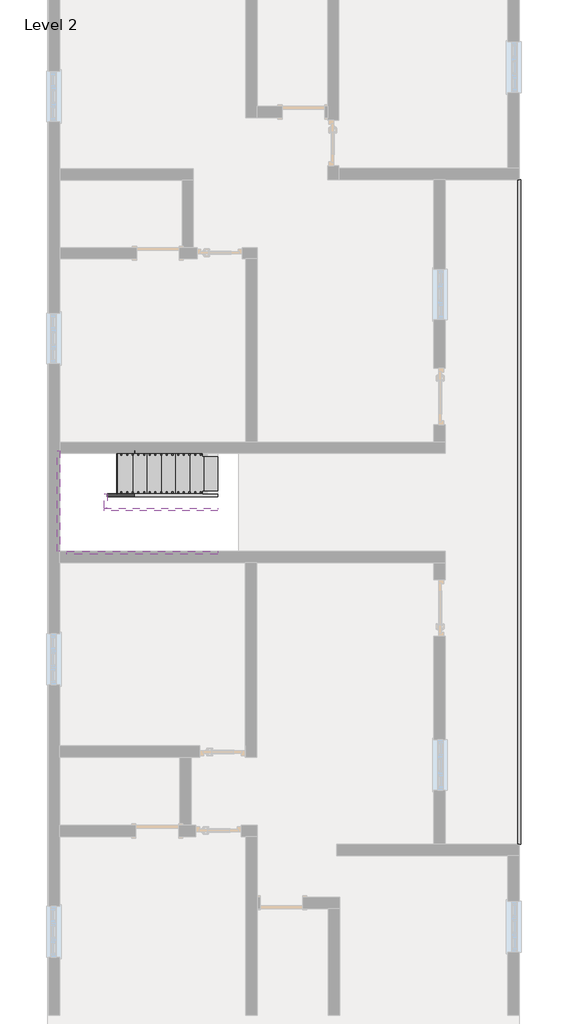
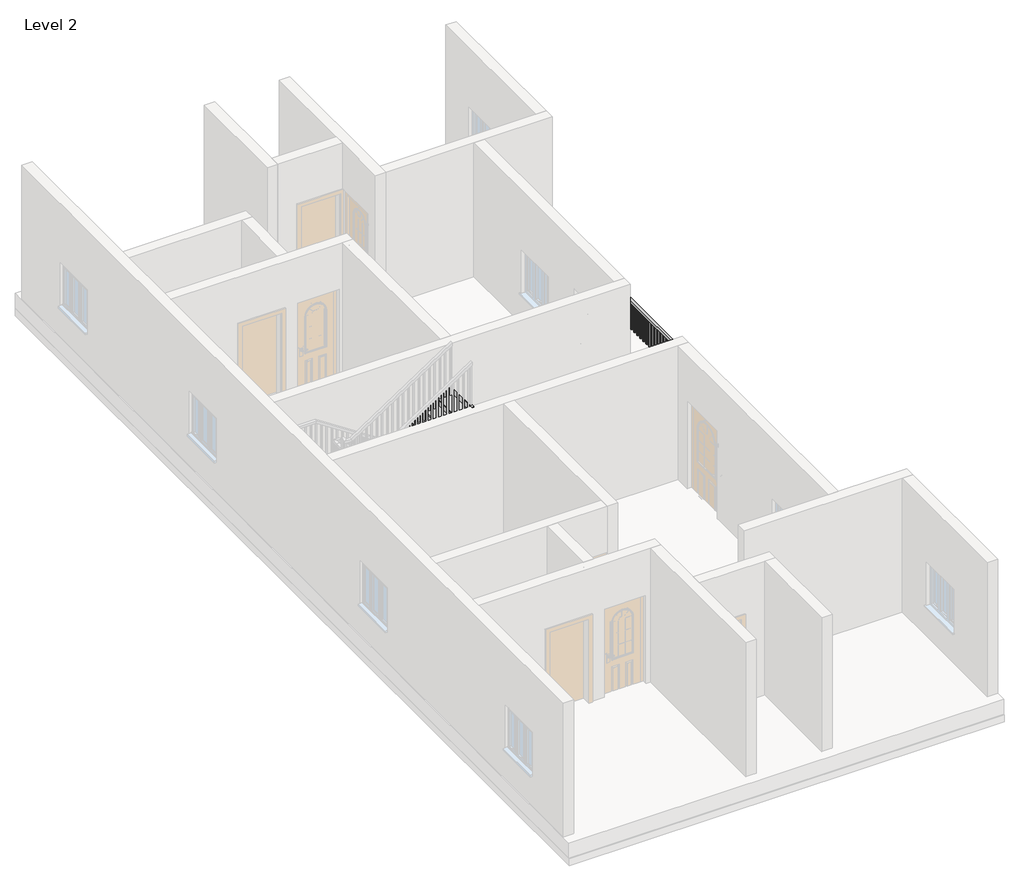
# One storey, part 3 of 3: 6 members, 1 railing, 1 stair flight.
"""IFC4 building model written with IfcOpenShell, lengths in millimetres."""

from ifc_helpers import new_model, si_unit, frame, origin, place, context, project, spatial, polyline, outline, extrude, transform, mapped, element, save
from components import stair_flight_1a1858fe

model = new_model("IFC4")

# Units and contexts
model_context = context("Model", 3, world=origin())
ifc_project = project(units=[si_unit("LENGTHUNIT", "METRE", prefix="MILLI")], contexts=[model_context])

# Site, building, storey
site = spatial("IfcSite", under=ifc_project)
building = spatial("IfcBuilding", under=site)
storey = spatial("IfcBuildingStorey", under=building, Name="Level 2", Elevation=3048.0)

# Members
placement = place(None, origin())
element("IfcMember", 1, ObjectType="Stringer - 2\" Width", at=placement, inside=storey, context=model_context, shape_type="SweptSolid", body=[
    extrude(outline(polyline([(3048.0, -2118.1728655), (3265.4747739, -2118.1728655), (4575.2681072, -4099.3728655), (4209.8806735, -4099.3728655), (3048.0, -2341.9063005), (3048.0, -2118.1728655)])), frame((0.0, 417.8797121, 0.0), z_axis=(0.0, 1.0, 0.0), x_axis=(0.0, 0.0, 1.0)), (0.0, 0.0, 1.0), 50.8),
])
element("IfcMember", 2, ObjectType="Stringer - 2\" Width", at=placement, inside=storey, context=model_context, shape_type="SweptSolid", body=[
    extrude(outline(polyline([(-4150.1728655, 468.6797121), (-4099.3728655, 468.6797121), (-4099.3728655, 214.6797121), (-4150.1728655, 214.6797121), (-4150.1728655, 468.6797121)])), frame((0.0, 0.0, 4330.7), z_axis=(0.0, 0.0, 1.0), x_axis=(1.0, 0.0, 0.0)), (0.0, 0.0, 1.0), 304.8),
])
element("IfcMember", 3, ObjectType="Stringer - 2\" Width", at=placement, inside=storey, context=model_context, shape_type="SweptSolid", body=[
    extrude(outline(polyline([(4776.7747739, -4150.1728655), (4411.3873402, -4150.1728655), (5754.765118, -2118.1728655), (6120.1525517, -2118.1728655), (4776.7747739, -4150.1728655)])), frame((0.0, 163.8797121, 0.0), z_axis=(0.0, 1.0, 0.0), x_axis=(0.0, 0.0, 1.0)), (0.0, 0.0, 1.0), 50.8),
])
element("IfcMember", 4, ObjectType="Stringer - 2\" Width", at=placement, inside=storey, context=model_context, shape_type="SweptSolid", body=[
    extrude(outline(polyline([(3048.0, -2118.1728655), (3265.4747739, -2118.1728655), (4635.5, -4190.4799301), (4635.5, -4743.1668047), (3048.0, -2341.9063005), (3048.0, -2118.1728655)])), frame((0.0, 1192.5797121, 0.0), z_axis=(0.0, 1.0, 0.0), x_axis=(0.0, 0.0, 1.0)), (0.0, 0.0, 1.0), 50.8),
])
element("IfcMember", 5, ObjectType="Stringer - 2\" Width", at=placement, inside=storey, context=model_context, shape_type="SweptSolid", body=[
    extrude(outline(polyline([(-4994.7394105, 1243.3797121), (-4943.9394105, 1243.3797121), (-4943.9394105, -560.0202879), (-4994.7394105, -560.0202879), (-4994.7394105, 1243.3797121)])), frame((0.0, 0.0, 4330.7), z_axis=(0.0, 0.0, 1.0), x_axis=(1.0, 0.0, 0.0)), (0.0, 0.0, 1.0), 304.8),
])
element("IfcMember", 6, ObjectType="Stringer - 2\" Width", at=placement, inside=storey, context=model_context, shape_type="SweptSolid", body=[
    extrude(outline(polyline([(4330.7, -4272.2209431), (5754.765118, -2118.1728655), (6120.1525517, -2118.1728655), (4330.7, -4824.9078176), (4330.7, -4272.2209431)])), frame((0.0, -610.8202879, 0.0), z_axis=(0.0, 1.0, 0.0), x_axis=(0.0, 0.0, 1.0)), (0.0, 0.0, 1.0), 50.8),
])

# Railing
element("IfcRailing", 7, ObjectType="Handrail - Rectangular", at=placement, inside=storey, context=model_context, shape_type="SweptSolid", body=[
    extrude(outline(polyline([(3298.3605895, -5805.1202879), (3247.5605895, -5805.1202879), (3247.5605895, 6094.2483916), (3298.3605895, 6094.2483916), (3298.3605895, -5805.1202879)])), frame((0.0, 0.0, 3911.6), z_axis=(0.0, 0.0, 1.0), x_axis=(1.0, 0.0, 0.0)), (0.0, 0.0, 1.0), 50.8),
    extrude(outline(polyline([(3282.4855895, 6072.5547121), (3263.4355895, 6072.5547121), (3263.4355895, 6091.6047121), (3282.4855895, 6091.6047121), (3282.4855895, 6072.5547121)])), frame((0.0, 0.0, 3048.0), z_axis=(0.0, 0.0, 1.0), x_axis=(1.0, 0.0, 0.0)), (0.0, 0.0, 1.0), 863.6),
    extrude(outline(polyline([(3282.4855895, 5970.9547121), (3263.4355895, 5970.9547121), (3263.4355895, 5990.0047121), (3282.4855895, 5990.0047121), (3282.4855895, 5970.9547121)])), frame((0.0, 0.0, 3048.0), z_axis=(0.0, 0.0, 1.0), x_axis=(1.0, 0.0, 0.0)), (0.0, 0.0, 1.0), 863.6),
    extrude(outline(polyline([(3282.4855895, 5869.3547121), (3263.4355895, 5869.3547121), (3263.4355895, 5888.4047121), (3282.4855895, 5888.4047121), (3282.4855895, 5869.3547121)])), frame((0.0, 0.0, 3048.0), z_axis=(0.0, 0.0, 1.0), x_axis=(1.0, 0.0, 0.0)), (0.0, 0.0, 1.0), 863.6),
    extrude(outline(polyline([(3282.4855895, 5767.7547121), (3263.4355895, 5767.7547121), (3263.4355895, 5786.8047121), (3282.4855895, 5786.8047121), (3282.4855895, 5767.7547121)])), frame((0.0, 0.0, 3048.0), z_axis=(0.0, 0.0, 1.0), x_axis=(1.0, 0.0, 0.0)), (0.0, 0.0, 1.0), 863.6),
    extrude(outline(polyline([(3282.4855895, 5666.1547121), (3263.4355895, 5666.1547121), (3263.4355895, 5685.2047121), (3282.4855895, 5685.2047121), (3282.4855895, 5666.1547121)])), frame((0.0, 0.0, 3048.0), z_axis=(0.0, 0.0, 1.0), x_axis=(1.0, 0.0, 0.0)), (0.0, 0.0, 1.0), 863.6),
    extrude(outline(polyline([(3282.4855895, 5564.5547121), (3263.4355895, 5564.5547121), (3263.4355895, 5583.6047121), (3282.4855895, 5583.6047121), (3282.4855895, 5564.5547121)])), frame((0.0, 0.0, 3048.0), z_axis=(0.0, 0.0, 1.0), x_axis=(1.0, 0.0, 0.0)), (0.0, 0.0, 1.0), 863.6),
    extrude(outline(polyline([(3282.4855895, 5462.9547121), (3263.4355895, 5462.9547121), (3263.4355895, 5482.0047121), (3282.4855895, 5482.0047121), (3282.4855895, 5462.9547121)])), frame((0.0, 0.0, 3048.0), z_axis=(0.0, 0.0, 1.0), x_axis=(1.0, 0.0, 0.0)), (0.0, 0.0, 1.0), 863.6),
    extrude(outline(polyline([(3282.4855895, 5361.3547121), (3263.4355895, 5361.3547121), (3263.4355895, 5380.4047121), (3282.4855895, 5380.4047121), (3282.4855895, 5361.3547121)])), frame((0.0, 0.0, 3048.0), z_axis=(0.0, 0.0, 1.0), x_axis=(1.0, 0.0, 0.0)), (0.0, 0.0, 1.0), 863.6),
    extrude(outline(polyline([(3282.4855895, 5259.7547121), (3263.4355895, 5259.7547121), (3263.4355895, 5278.8047121), (3282.4855895, 5278.8047121), (3282.4855895, 5259.7547121)])), frame((0.0, 0.0, 3048.0), z_axis=(0.0, 0.0, 1.0), x_axis=(1.0, 0.0, 0.0)), (0.0, 0.0, 1.0), 863.6),
    extrude(outline(polyline([(3282.4855895, 5158.1547121), (3263.4355895, 5158.1547121), (3263.4355895, 5177.2047121), (3282.4855895, 5177.2047121), (3282.4855895, 5158.1547121)])), frame((0.0, 0.0, 3048.0), z_axis=(0.0, 0.0, 1.0), x_axis=(1.0, 0.0, 0.0)), (0.0, 0.0, 1.0), 863.6),
    extrude(outline(polyline([(3282.4855895, 5056.5547121), (3263.4355895, 5056.5547121), (3263.4355895, 5075.6047121), (3282.4855895, 5075.6047121), (3282.4855895, 5056.5547121)])), frame((0.0, 0.0, 3048.0), z_axis=(0.0, 0.0, 1.0), x_axis=(1.0, 0.0, 0.0)), (0.0, 0.0, 1.0), 863.6),
    extrude(outline(polyline([(3282.4855895, 4954.9547121), (3263.4355895, 4954.9547121), (3263.4355895, 4974.0047121), (3282.4855895, 4974.0047121), (3282.4855895, 4954.9547121)])), frame((0.0, 0.0, 3048.0), z_axis=(0.0, 0.0, 1.0), x_axis=(1.0, 0.0, 0.0)), (0.0, 0.0, 1.0), 863.6),
    extrude(outline(polyline([(3282.4855895, 4853.3547121), (3263.4355895, 4853.3547121), (3263.4355895, 4872.4047121), (3282.4855895, 4872.4047121), (3282.4855895, 4853.3547121)])), frame((0.0, 0.0, 3048.0), z_axis=(0.0, 0.0, 1.0), x_axis=(1.0, 0.0, 0.0)), (0.0, 0.0, 1.0), 863.6),
    extrude(outline(polyline([(3282.4855895, 4751.7547121), (3263.4355895, 4751.7547121), (3263.4355895, 4770.8047121), (3282.4855895, 4770.8047121), (3282.4855895, 4751.7547121)])), frame((0.0, 0.0, 3048.0), z_axis=(0.0, 0.0, 1.0), x_axis=(1.0, 0.0, 0.0)), (0.0, 0.0, 1.0), 863.6),
    extrude(outline(polyline([(3282.4855895, 4650.1547121), (3263.4355895, 4650.1547121), (3263.4355895, 4669.2047121), (3282.4855895, 4669.2047121), (3282.4855895, 4650.1547121)])), frame((0.0, 0.0, 3048.0), z_axis=(0.0, 0.0, 1.0), x_axis=(1.0, 0.0, 0.0)), (0.0, 0.0, 1.0), 863.6),
    extrude(outline(polyline([(3282.4855895, 4548.5547121), (3263.4355895, 4548.5547121), (3263.4355895, 4567.6047121), (3282.4855895, 4567.6047121), (3282.4855895, 4548.5547121)])), frame((0.0, 0.0, 3048.0), z_axis=(0.0, 0.0, 1.0), x_axis=(1.0, 0.0, 0.0)), (0.0, 0.0, 1.0), 863.6),
    extrude(outline(polyline([(3282.4855895, 4446.9547121), (3263.4355895, 4446.9547121), (3263.4355895, 4466.0047121), (3282.4855895, 4466.0047121), (3282.4855895, 4446.9547121)])), frame((0.0, 0.0, 3048.0), z_axis=(0.0, 0.0, 1.0), x_axis=(1.0, 0.0, 0.0)), (0.0, 0.0, 1.0), 863.6),
    extrude(outline(polyline([(3282.4855895, 4345.3547121), (3263.4355895, 4345.3547121), (3263.4355895, 4364.4047121), (3282.4855895, 4364.4047121), (3282.4855895, 4345.3547121)])), frame((0.0, 0.0, 3048.0), z_axis=(0.0, 0.0, 1.0), x_axis=(1.0, 0.0, 0.0)), (0.0, 0.0, 1.0), 863.6),
    extrude(outline(polyline([(3282.4855895, 4243.7547121), (3263.4355895, 4243.7547121), (3263.4355895, 4262.8047121), (3282.4855895, 4262.8047121), (3282.4855895, 4243.7547121)])), frame((0.0, 0.0, 3048.0), z_axis=(0.0, 0.0, 1.0), x_axis=(1.0, 0.0, 0.0)), (0.0, 0.0, 1.0), 863.6),
    extrude(outline(polyline([(3282.4855895, 4142.1547121), (3263.4355895, 4142.1547121), (3263.4355895, 4161.2047121), (3282.4855895, 4161.2047121), (3282.4855895, 4142.1547121)])), frame((0.0, 0.0, 3048.0), z_axis=(0.0, 0.0, 1.0), x_axis=(1.0, 0.0, 0.0)), (0.0, 0.0, 1.0), 863.6),
    extrude(outline(polyline([(3282.4855895, 4040.5547121), (3263.4355895, 4040.5547121), (3263.4355895, 4059.6047121), (3282.4855895, 4059.6047121), (3282.4855895, 4040.5547121)])), frame((0.0, 0.0, 3048.0), z_axis=(0.0, 0.0, 1.0), x_axis=(1.0, 0.0, 0.0)), (0.0, 0.0, 1.0), 863.6),
    extrude(outline(polyline([(3282.4855895, 3938.9547121), (3263.4355895, 3938.9547121), (3263.4355895, 3958.0047121), (3282.4855895, 3958.0047121), (3282.4855895, 3938.9547121)])), frame((0.0, 0.0, 3048.0), z_axis=(0.0, 0.0, 1.0), x_axis=(1.0, 0.0, 0.0)), (0.0, 0.0, 1.0), 863.6),
    extrude(outline(polyline([(3282.4855895, 3837.3547121), (3263.4355895, 3837.3547121), (3263.4355895, 3856.4047121), (3282.4855895, 3856.4047121), (3282.4855895, 3837.3547121)])), frame((0.0, 0.0, 3048.0), z_axis=(0.0, 0.0, 1.0), x_axis=(1.0, 0.0, 0.0)), (0.0, 0.0, 1.0), 863.6),
    extrude(outline(polyline([(3282.4855895, 3735.7547121), (3263.4355895, 3735.7547121), (3263.4355895, 3754.8047121), (3282.4855895, 3754.8047121), (3282.4855895, 3735.7547121)])), frame((0.0, 0.0, 3048.0), z_axis=(0.0, 0.0, 1.0), x_axis=(1.0, 0.0, 0.0)), (0.0, 0.0, 1.0), 863.6),
    extrude(outline(polyline([(3282.4855895, 3634.1547121), (3263.4355895, 3634.1547121), (3263.4355895, 3653.2047121), (3282.4855895, 3653.2047121), (3282.4855895, 3634.1547121)])), frame((0.0, 0.0, 3048.0), z_axis=(0.0, 0.0, 1.0), x_axis=(1.0, 0.0, 0.0)), (0.0, 0.0, 1.0), 863.6),
    extrude(outline(polyline([(3282.4855895, 3532.5547121), (3263.4355895, 3532.5547121), (3263.4355895, 3551.6047121), (3282.4855895, 3551.6047121), (3282.4855895, 3532.5547121)])), frame((0.0, 0.0, 3048.0), z_axis=(0.0, 0.0, 1.0), x_axis=(1.0, 0.0, 0.0)), (0.0, 0.0, 1.0), 863.6),
    extrude(outline(polyline([(3282.4855895, 3430.9547121), (3263.4355895, 3430.9547121), (3263.4355895, 3450.0047121), (3282.4855895, 3450.0047121), (3282.4855895, 3430.9547121)])), frame((0.0, 0.0, 3048.0), z_axis=(0.0, 0.0, 1.0), x_axis=(1.0, 0.0, 0.0)), (0.0, 0.0, 1.0), 863.6),
    extrude(outline(polyline([(3282.4855895, 3329.3547121), (3263.4355895, 3329.3547121), (3263.4355895, 3348.4047121), (3282.4855895, 3348.4047121), (3282.4855895, 3329.3547121)])), frame((0.0, 0.0, 3048.0), z_axis=(0.0, 0.0, 1.0), x_axis=(1.0, 0.0, 0.0)), (0.0, 0.0, 1.0), 863.6),
    extrude(outline(polyline([(3282.4855895, 3227.7547121), (3263.4355895, 3227.7547121), (3263.4355895, 3246.8047121), (3282.4855895, 3246.8047121), (3282.4855895, 3227.7547121)])), frame((0.0, 0.0, 3048.0), z_axis=(0.0, 0.0, 1.0), x_axis=(1.0, 0.0, 0.0)), (0.0, 0.0, 1.0), 863.6),
    extrude(outline(polyline([(3282.4855895, 3126.1547121), (3263.4355895, 3126.1547121), (3263.4355895, 3145.2047121), (3282.4855895, 3145.2047121), (3282.4855895, 3126.1547121)])), frame((0.0, 0.0, 3048.0), z_axis=(0.0, 0.0, 1.0), x_axis=(1.0, 0.0, 0.0)), (0.0, 0.0, 1.0), 863.6),
    extrude(outline(polyline([(3282.4855895, 3024.5547121), (3263.4355895, 3024.5547121), (3263.4355895, 3043.6047121), (3282.4855895, 3043.6047121), (3282.4855895, 3024.5547121)])), frame((0.0, 0.0, 3048.0), z_axis=(0.0, 0.0, 1.0), x_axis=(1.0, 0.0, 0.0)), (0.0, 0.0, 1.0), 863.6),
    extrude(outline(polyline([(3282.4855895, 2922.9547121), (3263.4355895, 2922.9547121), (3263.4355895, 2942.0047121), (3282.4855895, 2942.0047121), (3282.4855895, 2922.9547121)])), frame((0.0, 0.0, 3048.0), z_axis=(0.0, 0.0, 1.0), x_axis=(1.0, 0.0, 0.0)), (0.0, 0.0, 1.0), 863.6),
    extrude(outline(polyline([(3282.4855895, 2821.3547121), (3263.4355895, 2821.3547121), (3263.4355895, 2840.4047121), (3282.4855895, 2840.4047121), (3282.4855895, 2821.3547121)])), frame((0.0, 0.0, 3048.0), z_axis=(0.0, 0.0, 1.0), x_axis=(1.0, 0.0, 0.0)), (0.0, 0.0, 1.0), 863.6),
    extrude(outline(polyline([(3282.4855895, 2719.7547121), (3263.4355895, 2719.7547121), (3263.4355895, 2738.8047121), (3282.4855895, 2738.8047121), (3282.4855895, 2719.7547121)])), frame((0.0, 0.0, 3048.0), z_axis=(0.0, 0.0, 1.0), x_axis=(1.0, 0.0, 0.0)), (0.0, 0.0, 1.0), 863.6),
    extrude(outline(polyline([(3282.4855895, 2618.1547121), (3263.4355895, 2618.1547121), (3263.4355895, 2637.2047121), (3282.4855895, 2637.2047121), (3282.4855895, 2618.1547121)])), frame((0.0, 0.0, 3048.0), z_axis=(0.0, 0.0, 1.0), x_axis=(1.0, 0.0, 0.0)), (0.0, 0.0, 1.0), 863.6),
    extrude(outline(polyline([(3282.4855895, 2516.5547121), (3263.4355895, 2516.5547121), (3263.4355895, 2535.6047121), (3282.4855895, 2535.6047121), (3282.4855895, 2516.5547121)])), frame((0.0, 0.0, 3048.0), z_axis=(0.0, 0.0, 1.0), x_axis=(1.0, 0.0, 0.0)), (0.0, 0.0, 1.0), 863.6),
    extrude(outline(polyline([(3282.4855895, 2414.9547121), (3263.4355895, 2414.9547121), (3263.4355895, 2434.0047121), (3282.4855895, 2434.0047121), (3282.4855895, 2414.9547121)])), frame((0.0, 0.0, 3048.0), z_axis=(0.0, 0.0, 1.0), x_axis=(1.0, 0.0, 0.0)), (0.0, 0.0, 1.0), 863.6),
    extrude(outline(polyline([(3282.4855895, 2313.3547121), (3263.4355895, 2313.3547121), (3263.4355895, 2332.4047121), (3282.4855895, 2332.4047121), (3282.4855895, 2313.3547121)])), frame((0.0, 0.0, 3048.0), z_axis=(0.0, 0.0, 1.0), x_axis=(1.0, 0.0, 0.0)), (0.0, 0.0, 1.0), 863.6),
    extrude(outline(polyline([(3282.4855895, 2211.7547121), (3263.4355895, 2211.7547121), (3263.4355895, 2230.8047121), (3282.4855895, 2230.8047121), (3282.4855895, 2211.7547121)])), frame((0.0, 0.0, 3048.0), z_axis=(0.0, 0.0, 1.0), x_axis=(1.0, 0.0, 0.0)), (0.0, 0.0, 1.0), 863.6),
    extrude(outline(polyline([(3282.4855895, 2110.1547121), (3263.4355895, 2110.1547121), (3263.4355895, 2129.2047121), (3282.4855895, 2129.2047121), (3282.4855895, 2110.1547121)])), frame((0.0, 0.0, 3048.0), z_axis=(0.0, 0.0, 1.0), x_axis=(1.0, 0.0, 0.0)), (0.0, 0.0, 1.0), 863.6),
    extrude(outline(polyline([(3282.4855895, 2008.5547121), (3263.4355895, 2008.5547121), (3263.4355895, 2027.6047121), (3282.4855895, 2027.6047121), (3282.4855895, 2008.5547121)])), frame((0.0, 0.0, 3048.0), z_axis=(0.0, 0.0, 1.0), x_axis=(1.0, 0.0, 0.0)), (0.0, 0.0, 1.0), 863.6),
    extrude(outline(polyline([(3282.4855895, 1906.9547121), (3263.4355895, 1906.9547121), (3263.4355895, 1926.0047121), (3282.4855895, 1926.0047121), (3282.4855895, 1906.9547121)])), frame((0.0, 0.0, 3048.0), z_axis=(0.0, 0.0, 1.0), x_axis=(1.0, 0.0, 0.0)), (0.0, 0.0, 1.0), 863.6),
    extrude(outline(polyline([(3282.4855895, 1805.3547121), (3263.4355895, 1805.3547121), (3263.4355895, 1824.4047121), (3282.4855895, 1824.4047121), (3282.4855895, 1805.3547121)])), frame((0.0, 0.0, 3048.0), z_axis=(0.0, 0.0, 1.0), x_axis=(1.0, 0.0, 0.0)), (0.0, 0.0, 1.0), 863.6),
    extrude(outline(polyline([(3282.4855895, 1703.7547121), (3263.4355895, 1703.7547121), (3263.4355895, 1722.8047121), (3282.4855895, 1722.8047121), (3282.4855895, 1703.7547121)])), frame((0.0, 0.0, 3048.0), z_axis=(0.0, 0.0, 1.0), x_axis=(1.0, 0.0, 0.0)), (0.0, 0.0, 1.0), 863.6),
    extrude(outline(polyline([(3282.4855895, 1602.1547121), (3263.4355895, 1602.1547121), (3263.4355895, 1621.2047121), (3282.4855895, 1621.2047121), (3282.4855895, 1602.1547121)])), frame((0.0, 0.0, 3048.0), z_axis=(0.0, 0.0, 1.0), x_axis=(1.0, 0.0, 0.0)), (0.0, 0.0, 1.0), 863.6),
    extrude(outline(polyline([(3282.4855895, 1500.5547121), (3263.4355895, 1500.5547121), (3263.4355895, 1519.6047121), (3282.4855895, 1519.6047121), (3282.4855895, 1500.5547121)])), frame((0.0, 0.0, 3048.0), z_axis=(0.0, 0.0, 1.0), x_axis=(1.0, 0.0, 0.0)), (0.0, 0.0, 1.0), 863.6),
    extrude(outline(polyline([(3282.4855895, 1398.9547121), (3263.4355895, 1398.9547121), (3263.4355895, 1418.0047121), (3282.4855895, 1418.0047121), (3282.4855895, 1398.9547121)])), frame((0.0, 0.0, 3048.0), z_axis=(0.0, 0.0, 1.0), x_axis=(1.0, 0.0, 0.0)), (0.0, 0.0, 1.0), 863.6),
    extrude(outline(polyline([(3282.4855895, 1297.3547121), (3263.4355895, 1297.3547121), (3263.4355895, 1316.4047121), (3282.4855895, 1316.4047121), (3282.4855895, 1297.3547121)])), frame((0.0, 0.0, 3048.0), z_axis=(0.0, 0.0, 1.0), x_axis=(1.0, 0.0, 0.0)), (0.0, 0.0, 1.0), 863.6),
    extrude(outline(polyline([(3282.4855895, 1195.7547121), (3263.4355895, 1195.7547121), (3263.4355895, 1214.8047121), (3282.4855895, 1214.8047121), (3282.4855895, 1195.7547121)])), frame((0.0, 0.0, 3048.0), z_axis=(0.0, 0.0, 1.0), x_axis=(1.0, 0.0, 0.0)), (0.0, 0.0, 1.0), 863.6),
    extrude(outline(polyline([(3282.4855895, 1094.1547121), (3263.4355895, 1094.1547121), (3263.4355895, 1113.2047121), (3282.4855895, 1113.2047121), (3282.4855895, 1094.1547121)])), frame((0.0, 0.0, 3048.0), z_axis=(0.0, 0.0, 1.0), x_axis=(1.0, 0.0, 0.0)), (0.0, 0.0, 1.0), 863.6),
    extrude(outline(polyline([(3282.4855895, 992.5547121), (3263.4355895, 992.5547121), (3263.4355895, 1011.6047121), (3282.4855895, 1011.6047121), (3282.4855895, 992.5547121)])), frame((0.0, 0.0, 3048.0), z_axis=(0.0, 0.0, 1.0), x_axis=(1.0, 0.0, 0.0)), (0.0, 0.0, 1.0), 863.6),
    extrude(outline(polyline([(3282.4855895, 890.9547121), (3263.4355895, 890.9547121), (3263.4355895, 910.0047121), (3282.4855895, 910.0047121), (3282.4855895, 890.9547121)])), frame((0.0, 0.0, 3048.0), z_axis=(0.0, 0.0, 1.0), x_axis=(1.0, 0.0, 0.0)), (0.0, 0.0, 1.0), 863.6),
    extrude(outline(polyline([(3282.4855895, 789.3547121), (3263.4355895, 789.3547121), (3263.4355895, 808.4047121), (3282.4855895, 808.4047121), (3282.4855895, 789.3547121)])), frame((0.0, 0.0, 3048.0), z_axis=(0.0, 0.0, 1.0), x_axis=(1.0, 0.0, 0.0)), (0.0, 0.0, 1.0), 863.6),
    extrude(outline(polyline([(3282.4855895, 687.7547121), (3263.4355895, 687.7547121), (3263.4355895, 706.8047121), (3282.4855895, 706.8047121), (3282.4855895, 687.7547121)])), frame((0.0, 0.0, 3048.0), z_axis=(0.0, 0.0, 1.0), x_axis=(1.0, 0.0, 0.0)), (0.0, 0.0, 1.0), 863.6),
    extrude(outline(polyline([(3282.4855895, 586.1547121), (3263.4355895, 586.1547121), (3263.4355895, 605.2047121), (3282.4855895, 605.2047121), (3282.4855895, 586.1547121)])), frame((0.0, 0.0, 3048.0), z_axis=(0.0, 0.0, 1.0), x_axis=(1.0, 0.0, 0.0)), (0.0, 0.0, 1.0), 863.6),
    extrude(outline(polyline([(3282.4855895, 484.5547121), (3263.4355895, 484.5547121), (3263.4355895, 503.6047121), (3282.4855895, 503.6047121), (3282.4855895, 484.5547121)])), frame((0.0, 0.0, 3048.0), z_axis=(0.0, 0.0, 1.0), x_axis=(1.0, 0.0, 0.0)), (0.0, 0.0, 1.0), 863.6),
    extrude(outline(polyline([(3282.4855895, 382.9547121), (3263.4355895, 382.9547121), (3263.4355895, 402.0047121), (3282.4855895, 402.0047121), (3282.4855895, 382.9547121)])), frame((0.0, 0.0, 3048.0), z_axis=(0.0, 0.0, 1.0), x_axis=(1.0, 0.0, 0.0)), (0.0, 0.0, 1.0), 863.6),
    extrude(outline(polyline([(3282.4855895, 281.3547121), (3263.4355895, 281.3547121), (3263.4355895, 300.4047121), (3282.4855895, 300.4047121), (3282.4855895, 281.3547121)])), frame((0.0, 0.0, 3048.0), z_axis=(0.0, 0.0, 1.0), x_axis=(1.0, 0.0, 0.0)), (0.0, 0.0, 1.0), 863.6),
    extrude(outline(polyline([(3282.4855895, 179.7547121), (3263.4355895, 179.7547121), (3263.4355895, 198.8047121), (3282.4855895, 198.8047121), (3282.4855895, 179.7547121)])), frame((0.0, 0.0, 3048.0), z_axis=(0.0, 0.0, 1.0), x_axis=(1.0, 0.0, 0.0)), (0.0, 0.0, 1.0), 863.6),
    extrude(outline(polyline([(3282.4855895, 78.1547121), (3263.4355895, 78.1547121), (3263.4355895, 97.2047121), (3282.4855895, 97.2047121), (3282.4855895, 78.1547121)])), frame((0.0, 0.0, 3048.0), z_axis=(0.0, 0.0, 1.0), x_axis=(1.0, 0.0, 0.0)), (0.0, 0.0, 1.0), 863.6),
    extrude(outline(polyline([(3282.4855895, -23.4452879), (3263.4355895, -23.4452879), (3263.4355895, -4.3952879), (3282.4855895, -4.3952879), (3282.4855895, -23.4452879)])), frame((0.0, 0.0, 3048.0), z_axis=(0.0, 0.0, 1.0), x_axis=(1.0, 0.0, 0.0)), (0.0, 0.0, 1.0), 863.6),
    extrude(outline(polyline([(3282.4855895, -125.0452879), (3263.4355895, -125.0452879), (3263.4355895, -105.9952879), (3282.4855895, -105.9952879), (3282.4855895, -125.0452879)])), frame((0.0, 0.0, 3048.0), z_axis=(0.0, 0.0, 1.0), x_axis=(1.0, 0.0, 0.0)), (0.0, 0.0, 1.0), 863.6),
    extrude(outline(polyline([(3282.4855895, -226.6452879), (3263.4355895, -226.6452879), (3263.4355895, -207.5952879), (3282.4855895, -207.5952879), (3282.4855895, -226.6452879)])), frame((0.0, 0.0, 3048.0), z_axis=(0.0, 0.0, 1.0), x_axis=(1.0, 0.0, 0.0)), (0.0, 0.0, 1.0), 863.6),
    extrude(outline(polyline([(3282.4855895, -328.2452879), (3263.4355895, -328.2452879), (3263.4355895, -309.1952879), (3282.4855895, -309.1952879), (3282.4855895, -328.2452879)])), frame((0.0, 0.0, 3048.0), z_axis=(0.0, 0.0, 1.0), x_axis=(1.0, 0.0, 0.0)), (0.0, 0.0, 1.0), 863.6),
    extrude(outline(polyline([(3282.4855895, -429.8452879), (3263.4355895, -429.8452879), (3263.4355895, -410.7952879), (3282.4855895, -410.7952879), (3282.4855895, -429.8452879)])), frame((0.0, 0.0, 3048.0), z_axis=(0.0, 0.0, 1.0), x_axis=(1.0, 0.0, 0.0)), (0.0, 0.0, 1.0), 863.6),
    extrude(outline(polyline([(3282.4855895, -531.4452879), (3263.4355895, -531.4452879), (3263.4355895, -512.3952879), (3282.4855895, -512.3952879), (3282.4855895, -531.4452879)])), frame((0.0, 0.0, 3048.0), z_axis=(0.0, 0.0, 1.0), x_axis=(1.0, 0.0, 0.0)), (0.0, 0.0, 1.0), 863.6),
    extrude(outline(polyline([(3282.4855895, -633.0452879), (3263.4355895, -633.0452879), (3263.4355895, -613.9952879), (3282.4855895, -613.9952879), (3282.4855895, -633.0452879)])), frame((0.0, 0.0, 3048.0), z_axis=(0.0, 0.0, 1.0), x_axis=(1.0, 0.0, 0.0)), (0.0, 0.0, 1.0), 863.6),
    extrude(outline(polyline([(3282.4855895, -734.6452879), (3263.4355895, -734.6452879), (3263.4355895, -715.5952879), (3282.4855895, -715.5952879), (3282.4855895, -734.6452879)])), frame((0.0, 0.0, 3048.0), z_axis=(0.0, 0.0, 1.0), x_axis=(1.0, 0.0, 0.0)), (0.0, 0.0, 1.0), 863.6),
    extrude(outline(polyline([(3282.4855895, -836.2452879), (3263.4355895, -836.2452879), (3263.4355895, -817.1952879), (3282.4855895, -817.1952879), (3282.4855895, -836.2452879)])), frame((0.0, 0.0, 3048.0), z_axis=(0.0, 0.0, 1.0), x_axis=(1.0, 0.0, 0.0)), (0.0, 0.0, 1.0), 863.6),
    extrude(outline(polyline([(3282.4855895, -937.8452879), (3263.4355895, -937.8452879), (3263.4355895, -918.7952879), (3282.4855895, -918.7952879), (3282.4855895, -937.8452879)])), frame((0.0, 0.0, 3048.0), z_axis=(0.0, 0.0, 1.0), x_axis=(1.0, 0.0, 0.0)), (0.0, 0.0, 1.0), 863.6),
    extrude(outline(polyline([(3282.4855895, -1039.4452879), (3263.4355895, -1039.4452879), (3263.4355895, -1020.3952879), (3282.4855895, -1020.3952879), (3282.4855895, -1039.4452879)])), frame((0.0, 0.0, 3048.0), z_axis=(0.0, 0.0, 1.0), x_axis=(1.0, 0.0, 0.0)), (0.0, 0.0, 1.0), 863.6),
    extrude(outline(polyline([(3282.4855895, -1141.0452879), (3263.4355895, -1141.0452879), (3263.4355895, -1121.9952879), (3282.4855895, -1121.9952879), (3282.4855895, -1141.0452879)])), frame((0.0, 0.0, 3048.0), z_axis=(0.0, 0.0, 1.0), x_axis=(1.0, 0.0, 0.0)), (0.0, 0.0, 1.0), 863.6),
    extrude(outline(polyline([(3282.4855895, -1242.6452879), (3263.4355895, -1242.6452879), (3263.4355895, -1223.5952879), (3282.4855895, -1223.5952879), (3282.4855895, -1242.6452879)])), frame((0.0, 0.0, 3048.0), z_axis=(0.0, 0.0, 1.0), x_axis=(1.0, 0.0, 0.0)), (0.0, 0.0, 1.0), 863.6),
    extrude(outline(polyline([(3282.4855895, -1344.2452879), (3263.4355895, -1344.2452879), (3263.4355895, -1325.1952879), (3282.4855895, -1325.1952879), (3282.4855895, -1344.2452879)])), frame((0.0, 0.0, 3048.0), z_axis=(0.0, 0.0, 1.0), x_axis=(1.0, 0.0, 0.0)), (0.0, 0.0, 1.0), 863.6),
    extrude(outline(polyline([(3282.4855895, -1445.8452879), (3263.4355895, -1445.8452879), (3263.4355895, -1426.7952879), (3282.4855895, -1426.7952879), (3282.4855895, -1445.8452879)])), frame((0.0, 0.0, 3048.0), z_axis=(0.0, 0.0, 1.0), x_axis=(1.0, 0.0, 0.0)), (0.0, 0.0, 1.0), 863.6),
    extrude(outline(polyline([(3282.4855895, -1547.4452879), (3263.4355895, -1547.4452879), (3263.4355895, -1528.3952879), (3282.4855895, -1528.3952879), (3282.4855895, -1547.4452879)])), frame((0.0, 0.0, 3048.0), z_axis=(0.0, 0.0, 1.0), x_axis=(1.0, 0.0, 0.0)), (0.0, 0.0, 1.0), 863.6),
    extrude(outline(polyline([(3282.4855895, -1649.0452879), (3263.4355895, -1649.0452879), (3263.4355895, -1629.9952879), (3282.4855895, -1629.9952879), (3282.4855895, -1649.0452879)])), frame((0.0, 0.0, 3048.0), z_axis=(0.0, 0.0, 1.0), x_axis=(1.0, 0.0, 0.0)), (0.0, 0.0, 1.0), 863.6),
    extrude(outline(polyline([(3282.4855895, -1750.6452879), (3263.4355895, -1750.6452879), (3263.4355895, -1731.5952879), (3282.4855895, -1731.5952879), (3282.4855895, -1750.6452879)])), frame((0.0, 0.0, 3048.0), z_axis=(0.0, 0.0, 1.0), x_axis=(1.0, 0.0, 0.0)), (0.0, 0.0, 1.0), 863.6),
    extrude(outline(polyline([(3282.4855895, -1852.2452879), (3263.4355895, -1852.2452879), (3263.4355895, -1833.1952879), (3282.4855895, -1833.1952879), (3282.4855895, -1852.2452879)])), frame((0.0, 0.0, 3048.0), z_axis=(0.0, 0.0, 1.0), x_axis=(1.0, 0.0, 0.0)), (0.0, 0.0, 1.0), 863.6),
    extrude(outline(polyline([(3282.4855895, -1953.8452879), (3263.4355895, -1953.8452879), (3263.4355895, -1934.7952879), (3282.4855895, -1934.7952879), (3282.4855895, -1953.8452879)])), frame((0.0, 0.0, 3048.0), z_axis=(0.0, 0.0, 1.0), x_axis=(1.0, 0.0, 0.0)), (0.0, 0.0, 1.0), 863.6),
    extrude(outline(polyline([(3282.4855895, -2055.4452879), (3263.4355895, -2055.4452879), (3263.4355895, -2036.3952879), (3282.4855895, -2036.3952879), (3282.4855895, -2055.4452879)])), frame((0.0, 0.0, 3048.0), z_axis=(0.0, 0.0, 1.0), x_axis=(1.0, 0.0, 0.0)), (0.0, 0.0, 1.0), 863.6),
    extrude(outline(polyline([(3282.4855895, -2157.0452879), (3263.4355895, -2157.0452879), (3263.4355895, -2137.9952879), (3282.4855895, -2137.9952879), (3282.4855895, -2157.0452879)])), frame((0.0, 0.0, 3048.0), z_axis=(0.0, 0.0, 1.0), x_axis=(1.0, 0.0, 0.0)), (0.0, 0.0, 1.0), 863.6),
    extrude(outline(polyline([(3282.4855895, -2258.6452879), (3263.4355895, -2258.6452879), (3263.4355895, -2239.5952879), (3282.4855895, -2239.5952879), (3282.4855895, -2258.6452879)])), frame((0.0, 0.0, 3048.0), z_axis=(0.0, 0.0, 1.0), x_axis=(1.0, 0.0, 0.0)), (0.0, 0.0, 1.0), 863.6),
    extrude(outline(polyline([(3282.4855895, -2360.2452879), (3263.4355895, -2360.2452879), (3263.4355895, -2341.1952879), (3282.4855895, -2341.1952879), (3282.4855895, -2360.2452879)])), frame((0.0, 0.0, 3048.0), z_axis=(0.0, 0.0, 1.0), x_axis=(1.0, 0.0, 0.0)), (0.0, 0.0, 1.0), 863.6),
    extrude(outline(polyline([(3282.4855895, -2461.8452879), (3263.4355895, -2461.8452879), (3263.4355895, -2442.7952879), (3282.4855895, -2442.7952879), (3282.4855895, -2461.8452879)])), frame((0.0, 0.0, 3048.0), z_axis=(0.0, 0.0, 1.0), x_axis=(1.0, 0.0, 0.0)), (0.0, 0.0, 1.0), 863.6),
    extrude(outline(polyline([(3282.4855895, -2563.4452879), (3263.4355895, -2563.4452879), (3263.4355895, -2544.3952879), (3282.4855895, -2544.3952879), (3282.4855895, -2563.4452879)])), frame((0.0, 0.0, 3048.0), z_axis=(0.0, 0.0, 1.0), x_axis=(1.0, 0.0, 0.0)), (0.0, 0.0, 1.0), 863.6),
    extrude(outline(polyline([(3282.4855895, -2665.0452879), (3263.4355895, -2665.0452879), (3263.4355895, -2645.9952879), (3282.4855895, -2645.9952879), (3282.4855895, -2665.0452879)])), frame((0.0, 0.0, 3048.0), z_axis=(0.0, 0.0, 1.0), x_axis=(1.0, 0.0, 0.0)), (0.0, 0.0, 1.0), 863.6),
    extrude(outline(polyline([(3282.4855895, -2766.6452879), (3263.4355895, -2766.6452879), (3263.4355895, -2747.5952879), (3282.4855895, -2747.5952879), (3282.4855895, -2766.6452879)])), frame((0.0, 0.0, 3048.0), z_axis=(0.0, 0.0, 1.0), x_axis=(1.0, 0.0, 0.0)), (0.0, 0.0, 1.0), 863.6),
    extrude(outline(polyline([(3282.4855895, -2868.2452879), (3263.4355895, -2868.2452879), (3263.4355895, -2849.1952879), (3282.4855895, -2849.1952879), (3282.4855895, -2868.2452879)])), frame((0.0, 0.0, 3048.0), z_axis=(0.0, 0.0, 1.0), x_axis=(1.0, 0.0, 0.0)), (0.0, 0.0, 1.0), 863.6),
    extrude(outline(polyline([(3282.4855895, -2969.8452879), (3263.4355895, -2969.8452879), (3263.4355895, -2950.7952879), (3282.4855895, -2950.7952879), (3282.4855895, -2969.8452879)])), frame((0.0, 0.0, 3048.0), z_axis=(0.0, 0.0, 1.0), x_axis=(1.0, 0.0, 0.0)), (0.0, 0.0, 1.0), 863.6),
    extrude(outline(polyline([(3282.4855895, -3071.4452879), (3263.4355895, -3071.4452879), (3263.4355895, -3052.3952879), (3282.4855895, -3052.3952879), (3282.4855895, -3071.4452879)])), frame((0.0, 0.0, 3048.0), z_axis=(0.0, 0.0, 1.0), x_axis=(1.0, 0.0, 0.0)), (0.0, 0.0, 1.0), 863.6),
    extrude(outline(polyline([(3282.4855895, -3173.0452879), (3263.4355895, -3173.0452879), (3263.4355895, -3153.9952879), (3282.4855895, -3153.9952879), (3282.4855895, -3173.0452879)])), frame((0.0, 0.0, 3048.0), z_axis=(0.0, 0.0, 1.0), x_axis=(1.0, 0.0, 0.0)), (0.0, 0.0, 1.0), 863.6),
    extrude(outline(polyline([(3282.4855895, -3274.6452879), (3263.4355895, -3274.6452879), (3263.4355895, -3255.5952879), (3282.4855895, -3255.5952879), (3282.4855895, -3274.6452879)])), frame((0.0, 0.0, 3048.0), z_axis=(0.0, 0.0, 1.0), x_axis=(1.0, 0.0, 0.0)), (0.0, 0.0, 1.0), 863.6),
    extrude(outline(polyline([(3282.4855895, -3376.2452879), (3263.4355895, -3376.2452879), (3263.4355895, -3357.1952879), (3282.4855895, -3357.1952879), (3282.4855895, -3376.2452879)])), frame((0.0, 0.0, 3048.0), z_axis=(0.0, 0.0, 1.0), x_axis=(1.0, 0.0, 0.0)), (0.0, 0.0, 1.0), 863.6),
    extrude(outline(polyline([(3282.4855895, -3477.8452879), (3263.4355895, -3477.8452879), (3263.4355895, -3458.7952879), (3282.4855895, -3458.7952879), (3282.4855895, -3477.8452879)])), frame((0.0, 0.0, 3048.0), z_axis=(0.0, 0.0, 1.0), x_axis=(1.0, 0.0, 0.0)), (0.0, 0.0, 1.0), 863.6),
    extrude(outline(polyline([(3282.4855895, -3579.4452879), (3263.4355895, -3579.4452879), (3263.4355895, -3560.3952879), (3282.4855895, -3560.3952879), (3282.4855895, -3579.4452879)])), frame((0.0, 0.0, 3048.0), z_axis=(0.0, 0.0, 1.0), x_axis=(1.0, 0.0, 0.0)), (0.0, 0.0, 1.0), 863.6),
    extrude(outline(polyline([(3282.4855895, -3681.0452879), (3263.4355895, -3681.0452879), (3263.4355895, -3661.9952879), (3282.4855895, -3661.9952879), (3282.4855895, -3681.0452879)])), frame((0.0, 0.0, 3048.0), z_axis=(0.0, 0.0, 1.0), x_axis=(1.0, 0.0, 0.0)), (0.0, 0.0, 1.0), 863.6),
    extrude(outline(polyline([(3282.4855895, -3782.6452879), (3263.4355895, -3782.6452879), (3263.4355895, -3763.5952879), (3282.4855895, -3763.5952879), (3282.4855895, -3782.6452879)])), frame((0.0, 0.0, 3048.0), z_axis=(0.0, 0.0, 1.0), x_axis=(1.0, 0.0, 0.0)), (0.0, 0.0, 1.0), 863.6),
    extrude(outline(polyline([(3282.4855895, -3884.2452879), (3263.4355895, -3884.2452879), (3263.4355895, -3865.1952879), (3282.4855895, -3865.1952879), (3282.4855895, -3884.2452879)])), frame((0.0, 0.0, 3048.0), z_axis=(0.0, 0.0, 1.0), x_axis=(1.0, 0.0, 0.0)), (0.0, 0.0, 1.0), 863.6),
    extrude(outline(polyline([(3282.4855895, -3985.8452879), (3263.4355895, -3985.8452879), (3263.4355895, -3966.7952879), (3282.4855895, -3966.7952879), (3282.4855895, -3985.8452879)])), frame((0.0, 0.0, 3048.0), z_axis=(0.0, 0.0, 1.0), x_axis=(1.0, 0.0, 0.0)), (0.0, 0.0, 1.0), 863.6),
    extrude(outline(polyline([(3282.4855895, -4087.4452879), (3263.4355895, -4087.4452879), (3263.4355895, -4068.3952879), (3282.4855895, -4068.3952879), (3282.4855895, -4087.4452879)])), frame((0.0, 0.0, 3048.0), z_axis=(0.0, 0.0, 1.0), x_axis=(1.0, 0.0, 0.0)), (0.0, 0.0, 1.0), 863.6),
    extrude(outline(polyline([(3282.4855895, -4189.0452879), (3263.4355895, -4189.0452879), (3263.4355895, -4169.9952879), (3282.4855895, -4169.9952879), (3282.4855895, -4189.0452879)])), frame((0.0, 0.0, 3048.0), z_axis=(0.0, 0.0, 1.0), x_axis=(1.0, 0.0, 0.0)), (0.0, 0.0, 1.0), 863.6),
    extrude(outline(polyline([(3282.4855895, -4290.6452879), (3263.4355895, -4290.6452879), (3263.4355895, -4271.5952879), (3282.4855895, -4271.5952879), (3282.4855895, -4290.6452879)])), frame((0.0, 0.0, 3048.0), z_axis=(0.0, 0.0, 1.0), x_axis=(1.0, 0.0, 0.0)), (0.0, 0.0, 1.0), 863.6),
    extrude(outline(polyline([(3282.4855895, -4392.2452879), (3263.4355895, -4392.2452879), (3263.4355895, -4373.1952879), (3282.4855895, -4373.1952879), (3282.4855895, -4392.2452879)])), frame((0.0, 0.0, 3048.0), z_axis=(0.0, 0.0, 1.0), x_axis=(1.0, 0.0, 0.0)), (0.0, 0.0, 1.0), 863.6),
    extrude(outline(polyline([(3282.4855895, -4493.8452879), (3263.4355895, -4493.8452879), (3263.4355895, -4474.7952879), (3282.4855895, -4474.7952879), (3282.4855895, -4493.8452879)])), frame((0.0, 0.0, 3048.0), z_axis=(0.0, 0.0, 1.0), x_axis=(1.0, 0.0, 0.0)), (0.0, 0.0, 1.0), 863.6),
    extrude(outline(polyline([(3282.4855895, -4595.4452879), (3263.4355895, -4595.4452879), (3263.4355895, -4576.3952879), (3282.4855895, -4576.3952879), (3282.4855895, -4595.4452879)])), frame((0.0, 0.0, 3048.0), z_axis=(0.0, 0.0, 1.0), x_axis=(1.0, 0.0, 0.0)), (0.0, 0.0, 1.0), 863.6),
    extrude(outline(polyline([(3282.4855895, -4697.0452879), (3263.4355895, -4697.0452879), (3263.4355895, -4677.9952879), (3282.4855895, -4677.9952879), (3282.4855895, -4697.0452879)])), frame((0.0, 0.0, 3048.0), z_axis=(0.0, 0.0, 1.0), x_axis=(1.0, 0.0, 0.0)), (0.0, 0.0, 1.0), 863.6),
    extrude(outline(polyline([(3282.4855895, -4798.6452879), (3263.4355895, -4798.6452879), (3263.4355895, -4779.5952879), (3282.4855895, -4779.5952879), (3282.4855895, -4798.6452879)])), frame((0.0, 0.0, 3048.0), z_axis=(0.0, 0.0, 1.0), x_axis=(1.0, 0.0, 0.0)), (0.0, 0.0, 1.0), 863.6),
    extrude(outline(polyline([(3282.4855895, -4900.2452879), (3263.4355895, -4900.2452879), (3263.4355895, -4881.1952879), (3282.4855895, -4881.1952879), (3282.4855895, -4900.2452879)])), frame((0.0, 0.0, 3048.0), z_axis=(0.0, 0.0, 1.0), x_axis=(1.0, 0.0, 0.0)), (0.0, 0.0, 1.0), 863.6),
    extrude(outline(polyline([(3282.4855895, -5001.8452879), (3263.4355895, -5001.8452879), (3263.4355895, -4982.7952879), (3282.4855895, -4982.7952879), (3282.4855895, -5001.8452879)])), frame((0.0, 0.0, 3048.0), z_axis=(0.0, 0.0, 1.0), x_axis=(1.0, 0.0, 0.0)), (0.0, 0.0, 1.0), 863.6),
    extrude(outline(polyline([(3282.4855895, -5103.4452879), (3263.4355895, -5103.4452879), (3263.4355895, -5084.3952879), (3282.4855895, -5084.3952879), (3282.4855895, -5103.4452879)])), frame((0.0, 0.0, 3048.0), z_axis=(0.0, 0.0, 1.0), x_axis=(1.0, 0.0, 0.0)), (0.0, 0.0, 1.0), 863.6),
    extrude(outline(polyline([(3282.4855895, -5205.0452879), (3263.4355895, -5205.0452879), (3263.4355895, -5185.9952879), (3282.4855895, -5185.9952879), (3282.4855895, -5205.0452879)])), frame((0.0, 0.0, 3048.0), z_axis=(0.0, 0.0, 1.0), x_axis=(1.0, 0.0, 0.0)), (0.0, 0.0, 1.0), 863.6),
    extrude(outline(polyline([(3282.4855895, -5306.6452879), (3263.4355895, -5306.6452879), (3263.4355895, -5287.5952879), (3282.4855895, -5287.5952879), (3282.4855895, -5306.6452879)])), frame((0.0, 0.0, 3048.0), z_axis=(0.0, 0.0, 1.0), x_axis=(1.0, 0.0, 0.0)), (0.0, 0.0, 1.0), 863.6),
    extrude(outline(polyline([(3282.4855895, -5408.2452879), (3263.4355895, -5408.2452879), (3263.4355895, -5389.1952879), (3282.4855895, -5389.1952879), (3282.4855895, -5408.2452879)])), frame((0.0, 0.0, 3048.0), z_axis=(0.0, 0.0, 1.0), x_axis=(1.0, 0.0, 0.0)), (0.0, 0.0, 1.0), 863.6),
    extrude(outline(polyline([(3282.4855895, -5509.8452879), (3263.4355895, -5509.8452879), (3263.4355895, -5490.7952879), (3282.4855895, -5490.7952879), (3282.4855895, -5509.8452879)])), frame((0.0, 0.0, 3048.0), z_axis=(0.0, 0.0, 1.0), x_axis=(1.0, 0.0, 0.0)), (0.0, 0.0, 1.0), 863.6),
    extrude(outline(polyline([(3282.4855895, -5611.4452879), (3263.4355895, -5611.4452879), (3263.4355895, -5592.3952879), (3282.4855895, -5592.3952879), (3282.4855895, -5611.4452879)])), frame((0.0, 0.0, 3048.0), z_axis=(0.0, 0.0, 1.0), x_axis=(1.0, 0.0, 0.0)), (0.0, 0.0, 1.0), 863.6),
    extrude(outline(polyline([(3282.4855895, -5713.0452879), (3263.4355895, -5713.0452879), (3263.4355895, -5693.9952879), (3282.4855895, -5693.9952879), (3282.4855895, -5713.0452879)])), frame((0.0, 0.0, 3048.0), z_axis=(0.0, 0.0, 1.0), x_axis=(1.0, 0.0, 0.0)), (0.0, 0.0, 1.0), 863.6),
    extrude(outline(polyline([(3282.4855895, 6075.1983916), (3263.4355895, 6075.1983916), (3263.4355895, 6094.2483916), (3282.4855895, 6094.2483916), (3282.4855895, 6075.1983916)])), frame((0.0, 0.0, 3048.0), z_axis=(0.0, 0.0, 1.0), x_axis=(1.0, 0.0, 0.0)), (0.0, 0.0, 1.0), 863.6),
    extrude(outline(polyline([(3282.4855895, -5805.1202879), (3263.4355895, -5805.1202879), (3263.4355895, -5786.0702879), (3282.4855895, -5786.0702879), (3282.4855895, -5805.1202879)])), frame((0.0, 0.0, 3048.0), z_axis=(0.0, 0.0, 1.0), x_axis=(1.0, 0.0, 0.0)), (0.0, 0.0, 1.0), 863.6),
])

# Stair flight
stair_flight_shape = stair_flight_1a1858fe(model_context)
element("IfcStairFlight", 8, ObjectType="2\" Tread 1\" Nosing 1/4\" Riser", at=placement, inside=storey, context=model_context, shape_type="MappedRepresentation", body=[
    mapped(stair_flight_shape, transform((0.0, 0.0, 0.0), x_axis=(1.0, 0.0, 0.0), y_axis=(0.0, 1.0, 0.0), z_axis=(0.0, 0.0, 1.0))),
])

save(model, "model.ifc")

# Revit data of these elements
# Type "Handrail - Rectangular"
#   Assembly Code = "C2010400"
#   built-in parameter 1008612 = 0.0416667 (stored number, unit not read)
#   built-in parameter 1008611 = 0.0416667 (stored number, unit not read)
#   built-in parameter 1008609 = 0.333333 (stored number, unit not read)
#   built-in parameter 1008604 = 0.166667 (stored number, unit not read)
#   built-in parameter 1008603 = 0.166667 (stored number, unit not read)
#   Railing Height = 914.4 mm
#   built-in parameter 1008630 = 2
#   built-in parameter 1008610 = 2
#   built-in parameter 1008618 = Baluster - Square : 3/4"
# Elements 1, 2, 3, 4, 5, 6 (IfcMember, "Stringer - 2\" Width")
#   Phase Created = New Construction
# Element 7 (IfcRailing, "Handrail - Rectangular")
#   Phase Created = New Construction
# Element 8 (IfcStairFlight, "2\" Tread 1\" Nosing 1/4\" Riser")
#   Phase Created = New Construction
